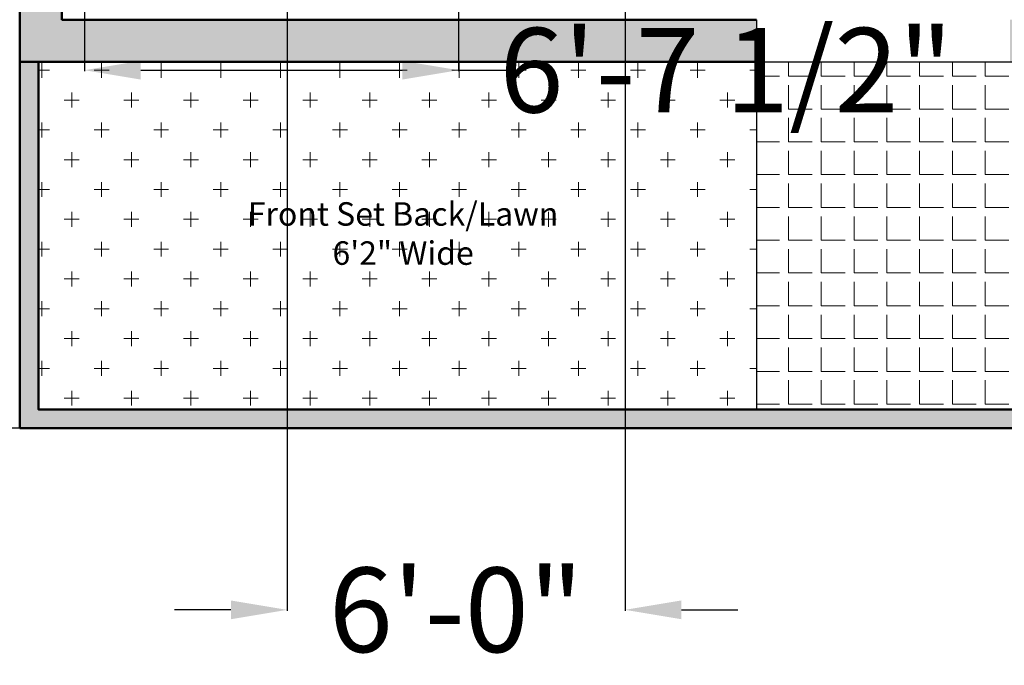
# Model space of a CAD drawing. Units: inches. Extents: x 2796 to 3603, y 978 to 1787.
# Tile 2 of 15: x 3070 to 3280, y 978 to 1116. Entities that reach past the tile are written whole.
import ezdxf

# ---------------------------------------------------------------- set-up
doc = ezdxf.new("R2010")
doc.units = ezdxf.units.IN
for name, color, linetype, lineweight in [('A-ANNO-DIMS', 7, 'Continuous', 18), ('A-AREA-IDEN', 7, 'Continuous', 18), ('A-WALL-EXTR-PATT', 1, 'Continuous', 13), ('L-PAVE', 1, 'Continuous', 25), ('L-PAVE-PATT', 7, 'Continuous', 13), ('L-PLNT-PATT', 7, 'Continuous', 13), ('Outer Wall', 1, 'Continuous', 50)]:
    doc.layers.add(name, color=color, linetype=linetype, lineweight=lineweight)
doc.styles.get("Standard").update_dxf_attribs({"font": 'arial.ttf'})
doc.dimstyles.get("Standard").update_dxf_attribs({"dimtxt": 18, "dimasz": 12, "dimexe": 0.18, "dimexo": 0.0625, "dimgap": 0.09, "dimtad": 0, "dimtih": 1, "dimtoh": 1, "dimdec": 0, "dimzin": 0, "dimdsep": 46, "dimlunit": 3, "dimtxsty": 'Standard', "dimcen": 0.09, "dimadec": 0, "dimazin": 0, "dimtfac": 1, "dimtdec": 0, "dimtofl": 0, "dimtmove": 0, "dimatfit": 3, "dimfxl": 1, "dimtolj": 1, "dimtzin": 0, "dimarcsym": 0})

# ---------------------------------------------------------------- blocks, each defined once
blk = doc.blocks.new('*D12')
at = {"layer": 'A-ANNO-DIMS', "color": 0, "lineweight": -2, "transparency": 16777216}
for p, q in [((3070.18, 1736.68), (3041.33, 1736.68)), ((3041.51, 1724.68), (3041.51, 1391.96)), ((3041.51, 1040.68), (3041.51, 1373.4)), ((3070.18, 1028.68), (3041.33, 1028.68))]:
    blk.add_line(p, q, dxfattribs=at)
at = {"layer": 'A-ANNO-DIMS', "color": 0, "transparency": 16777216}
for points in [[(3039.51, 1724.68), (3043.51, 1724.68), (3041.51, 1736.68)], [(3039.51, 1040.68), (3043.51, 1040.68), (3041.51, 1028.68)]]:
    blk.add_solid(points, dxfattribs=at)
at = {"layer": 'Defpoints', "color": 0, "transparency": 16777216}
for p in [(3041.51, 1736.68), (3070.25, 1736.68), (3070.25, 1028.68)]:
    blk.add_point(p, dxfattribs=at)
at = {"layer": 'A-ANNO-DIMS', "color": 0, "transparency": 16777216, "insert": (3041.51, 1382.68), "char_height": 18, "attachment_point": 5}
blk.add_mtext("\\A1;59'", dxfattribs=at)
blk = doc.blocks.new('*D31')
at = {"layer": 'A-ANNO-DIMS', "color": 0, "lineweight": -2, "transparency": 16777216}
for p, q in [((3084.05, 1128.75), (3084.05, 1104.74)), ((3163.77, 1128.75), (3163.77, 1104.74)), ((3096.05, 1104.92), (3151.77, 1104.92)), ((3163.77, 1104.92), (3175.77, 1104.92))]:
    blk.add_line(p, q, dxfattribs=at)
at = {"layer": 'A-ANNO-DIMS', "color": 0, "transparency": 16777216}
for points in [[(3096.05, 1106.92), (3096.05, 1102.92), (3084.05, 1104.92)], [(3151.77, 1106.92), (3151.77, 1102.92), (3163.77, 1104.92)]]:
    blk.add_solid(points, dxfattribs=at)
at = {"layer": 'Defpoints', "color": 0, "transparency": 16777216}
for p in [(3084.05, 1128.81), (3163.77, 1128.81), (3163.77, 1104.92)]:
    blk.add_point(p, dxfattribs=at)
at = {"layer": 'A-ANNO-DIMS', "color": 0, "transparency": 16777216, "insert": (3220.81, 1104.92), "char_height": 18, "attachment_point": 5}
blk.add_mtext('\\A1;6\'-7 1/2"', dxfattribs=at)
blk = doc.blocks.new('*D51')
at = {"layer": 'A-ANNO-DIMS', "color": 0, "lineweight": -2, "transparency": 16777216}
for p, q in [((3127.245499, 1431.61284), (3127.245499, 989.79534)), ((3199.245499, 1431.61284), (3199.245499, 989.79534)), ((3115.245499, 989.97534), (3103.245499, 989.97534)), ((3211.245499, 989.97534), (3223.245499, 989.97534))]:
    blk.add_line(p, q, dxfattribs=at)
at = {"layer": 'A-ANNO-DIMS', "color": 0, "transparency": 16777216}
for points in [[(3115.245499, 991.97534), (3115.245499, 987.97534), (3127.245499, 989.97534)], [(3211.245499, 991.97534), (3211.245499, 987.97534), (3199.245499, 989.97534)]]:
    blk.add_solid(points, dxfattribs=at)
at = {"layer": 'Defpoints', "color": 0, "transparency": 16777216}
for p in [(3127.245499, 1431.67534), (3199.245499, 1431.67534), (3199.245499, 989.97534)]:
    blk.add_point(p, dxfattribs=at)
at = {"layer": 'A-ANNO-DIMS', "color": 0, "transparency": 16777216, "insert": (3163.245499, 989.97534), "char_height": 18, "attachment_point": 5}
blk.add_mtext('\\A1;6\'-0"', dxfattribs=at)

msp = doc.modelspace()

# ---------------------------------------------------------------- hatches: boundary and pattern name
at = {"layer": 'A-WALL-EXTR-PATT'}
h = msp.add_hatch(color=256, dxfattribs=at)
h.dxf.hatch_style = 1
h.paths.add_polyline_path([(3424.25, 1736.68), (3070.25, 1736.68), (3070.25, 1106.68), (3227.25, 1106.68), (3227.25, 1115.68), (3226.75, 1115.68), (3223.75, 1115.68), (3079.25, 1115.68), (3079.25, 1727.68), (3127.25, 1727.68), (3415.25, 1727.68), (3415.25, 1188.68), (3424.25, 1188.68)])
h.paths.add_polyline_path([(3291.25, 1032.68), (3074.25, 1032.68), (3074.25, 1106.68), (3070.25, 1106.68), (3070.25, 1028.68), (3291.25, 1028.68)])
h.paths.add_polyline_path([(3291.25, 1115.68), (3281.25, 1115.68), (3281.25, 1106.68), (3291.25, 1106.68)], flags=17)
h.paths.add_polyline_path([(3301.25, 1037.68), (3291.25, 1037.68), (3291.25, 1028.68), (3301.25, 1028.68)])
h.paths.add_polyline_path([(3424.25, 1037.68), (3414.25, 1037.68), (3414.25, 1028.68), (3424.25, 1028.68)])
h.paths.add_polyline_path([(3424.25, 1188.68), (3420.25, 1188.68), (3420.25, 1037.68), (3424.25, 1037.68)])
at = {"layer": 'L-PAVE-PATT'}
h = msp.add_hatch(dxfattribs=at)
h.set_pattern_fill('ANGLE', color=256)
h.set_pattern_definition([(0, (0, 0), (0, 6.985), [5.08, -1.905]), (90, (0, 0), (-6.985, 4e-16), [5.08, -1.905])])
h.paths.add_polyline_path([(3291.25, 1106.68), (3227.25, 1106.68), (3227.25, 1032.68), (3291.25, 1032.68)])
at = {"layer": 'L-PLNT-PATT'}
h = msp.add_hatch(dxfattribs=at)
h.set_pattern_fill('CROSS', color=256)
h.paths.add_polyline_path([(3227.25, 1106.68), (3074.25, 1106.68), (3074.25, 1032.68), (3227.25, 1032.68)])
h.paths.add_polyline_path([(3119.08, 1060.37), (3184.73, 1060.37), (3184.73, 1079.51), (3119.08, 1079.51)], flags=24)

# ---------------------------------------------------------------- linework, layer by layer
at = {"layer": 'L-PAVE'}
for p, q in [((3227.25, 1115.68), (3227.25, 1032.68)), ((3227.25, 1106.68), (3291.25, 1106.68))]:
    msp.add_line(p, q, dxfattribs=at)
at = {"layer": 'Outer Wall'}
for p, q in [((3070.25, 1028.68), (3070.25, 1736.68)), ((3079.25, 1115.68), (3079.25, 1727.68)), ((3079.25, 1115.68), (3227.25, 1115.68)), ((3070.25, 1106.68), (3227.25, 1106.68)), ((3070.25, 1028.68), (3301.25, 1028.68))]:
    msp.add_line(p, q, dxfattribs=at)
msp.add_lwpolyline([(3291.25, 1032.68), (3074.25, 1032.68), (3074.25, 1106.68)], dxfattribs=at)

# ---------------------------------------------------------------- texts
at = {"layer": 'A-AREA-IDEN', "insert": (3195.31, 1076.8), "char_height": 5, "attachment_point": 3}
msp.add_mtext_dynamic_manual_height_columns('\\pxqc;{\\fTimes New Roman|b0|i0|c0|p18;Front Set Back/Lawn\\P6\'2" Wide}', width=86.7226, gutter_width=12.5, heights=[0], dxfattribs=at)

# ---------------------------------------------------------------- dimensions: what is measured, and where the dimension line sits
at = {"layer": 'A-ANNO-DIMS'}
dim = msp.add_linear_dim(base=(3041.51, 1736.68), p1=(3070.25, 1028.68), p2=(3070.25, 1736.68), angle=90, dimstyle='Standard', override={"dimclrd": 0, "dimclre": 0, "dimclrt": 0}, dxfattribs=at)
dim.commit()
dim.dimension.update_dxf_attribs({"geometry": '*D12', "text_midpoint": (3041.51, 1382.68)})
for base, p1, p2, picture, middle in [((3199.25, 989.98), (3127.25, 1431.68), (3199.25, 1431.68), '*D51', (3163.25, 989.98)), ((3163.77, 1104.92), (3084.05, 1128.81), (3163.77, 1128.81), '*D31', (3220.81, 1104.92))]:
    dim = msp.add_linear_dim(base=base, p1=p1, p2=p2, dimstyle='Standard', override={"dimdec": 1, "dimlfac": 1, "dimrnd": 0, "dimzin": 1, "dimdsep": 46, "dimlunit": 4, "dimfrac": 2}, dxfattribs=at)
    dim.commit()
    dim.dimension.update_dxf_attribs({"geometry": picture, "text_midpoint": middle})

doc.saveas('drawing.dxf')
